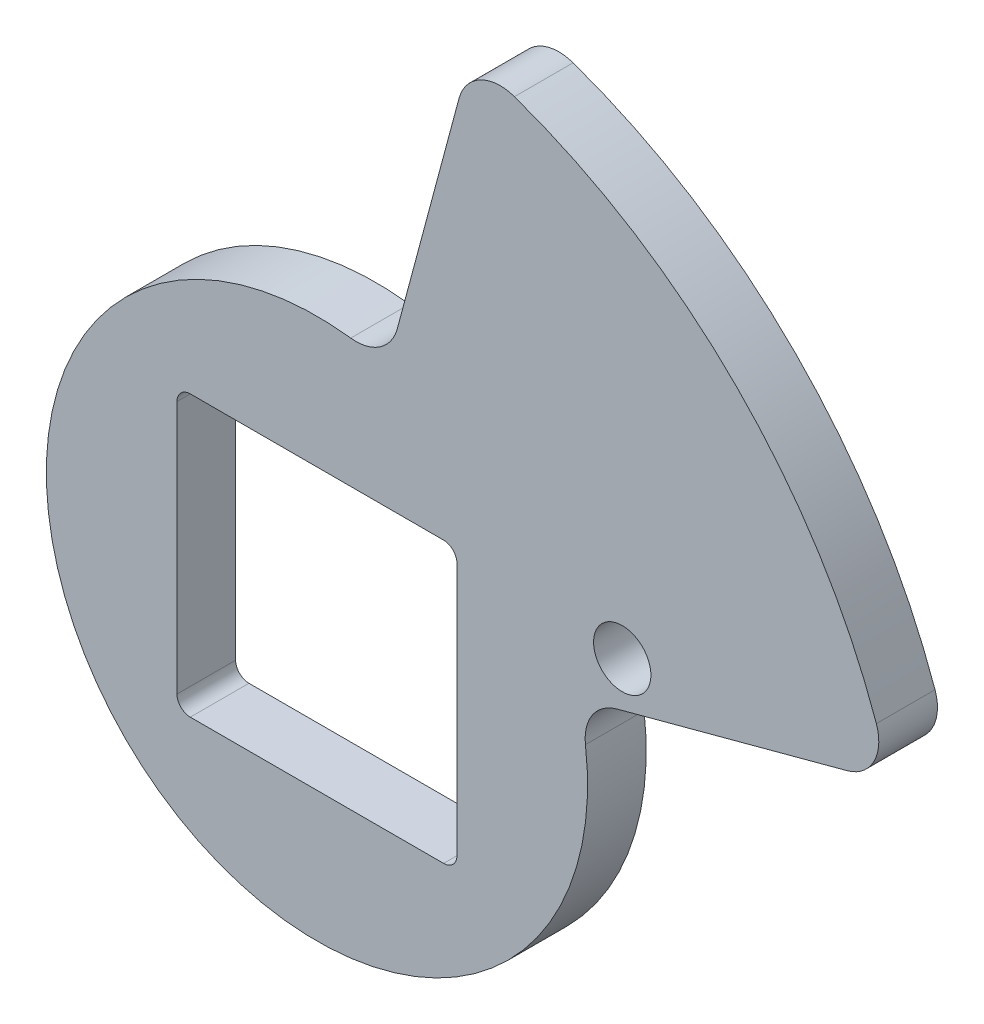
from build123d import *

# Parameters (mm, degrees)
LEVER_PLATE_4_4MM_DEPTH             = 4.4
SQUARE_DRIVE_AND_PIN_HOLE_SKETCH_R  = 2.15
SQUARE_DRIVE_AND_PIN_HOLE_CUT_DEPTH = 28.4


with BuildPart() as part:
    # Lever Plate Profile Sketch → Lever Plate 4.4mm (new body)
    with BuildSketch(Plane.XY):
        with BuildLine():
            Line((22.487823695, 6.025594199), (39.772809624, 10.65709222))
            ThreePointArc((39.772809624, 10.65709222), (41.775818518, 12.256700578), (41.962087077, 14.813279454))
            ThreePointArc((41.962087077, 14.813279454), (31.466251763, 31.466251763), (14.813279454, 41.962087077))
            ThreePointArc((14.813279454, 41.962087077), (12.256700578, 41.775818518), (10.65709222, 39.772809624))
            Line((10.65709222, 39.772809624), (6.025594199, 22.487823695))
            ThreePointArc((6.025594199, 22.487823695), (4.720025285, 20.660414916), (2.535022151, 20.14109388))
            ThreePointArc((2.535022151, 20.14109388), (-14.354267658, -14.354267658), (20.14109388, 2.535022151))
            ThreePointArc((20.14109388, 2.535022151), (20.660414916, 4.720025285), (22.487823695, 6.025594199))
        make_face()
    extrude(amount=LEVER_PLATE_4_4MM_DEPTH)

    # Square Drive and Pin Hole Sketch → Square Drive and Pin Hole Cut (cut)
    with BuildSketch(Plane.XY.offset(4.4)):
        with Locations((22.9, 9.5)):
            Circle(SQUARE_DRIVE_AND_PIN_HOLE_SKETCH_R)
        with BuildLine():
            Line((-10.5, 0), (-10.5, -9.5))
            ThreePointArc((-10.5, -9.5), (-10.207106781, -10.207106781), (-9.5, -10.5))
            Line((-9.5, -10.5), (9.5, -10.5))
            ThreePointArc((9.5, -10.5), (10.207106781, -10.207106781), (10.5, -9.5))
            Line((10.5, -9.5), (10.5, 9.5))
            ThreePointArc((10.5, 9.5), (10.207106781, 10.207106781), (9.5, 10.5))
            Line((9.5, 10.5), (-9.5, 10.5))
            ThreePointArc((-9.5, 10.5), (-10.207106781, 10.207106781), (-10.5, 9.5))
            Line((-10.5, 9.5), (-10.5, 0))
        make_face()
    extrude(amount=-SQUARE_DRIVE_AND_PIN_HOLE_CUT_DEPTH, mode=Mode.SUBTRACT)


solid = part.part
